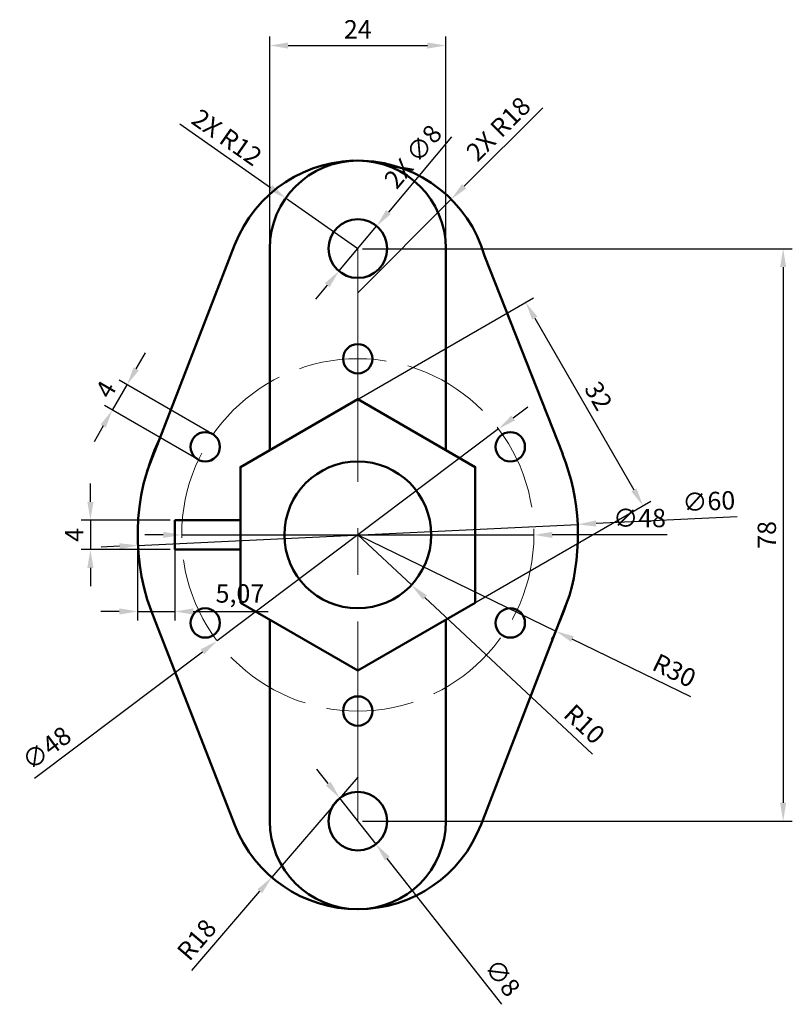
# Model space of a CAD drawing. Units: millimetres. Extents: x 3018 to 3124, y 2213 to 2348.
import ezdxf

# ---------------------------------------------------------------- set-up
doc = ezdxf.new("R2010")
doc.units = ezdxf.units.MM
doc.linetypes.add('ACAD_ISO02W100', pattern=[15, 12, -3])
doc.linetypes.add('CENTER', pattern=[50.8, 31.75, -6.35, 6.35, -6.35])
for name, color, linetype, lineweight in [('M-CNTR', 4, 'CENTER', 18), ('M-CNTR-PCD', 4, 'ACAD_ISO02W100', 18), ('M-DIMS', 2, 'Continuous', 25), ('M-OUTL', 7, 'Continuous', 50)]:
    doc.layers.add(name, color=color, linetype=linetype, lineweight=lineweight)
doc.styles.get("Standard").update_dxf_attribs({"font": 'arial.ttf'})
doc.dimstyles.new('ISO-25', dxfattribs={"dimtxt": 2.5, "dimasz": 2.5, "dimexe": 1.25, "dimexo": 0.625, "dimtad": 1, "dimtxsty": 'Standard', "dimcen": 2.5, "dimadec": 0, "dimazin": 0, "dimtfac": 1, "dimtmove": 0, "dimatfit": 3, "dimfxl": 1, "dimarcsym": 0})

# ---------------------------------------------------------------- blocks, each defined once
blk = doc.blocks.new('*D1')
at = {"layer": 'Defpoints', "color": 0, "transparency": 16777216}
for p in [(3056.3, 2291.27), (3103.18, 2281.39), (3072.3, 2263.56)]:
    blk.add_point(p, dxfattribs=at)
at = {"layer": 'M-DIMS', "color": 0, "lineweight": -2, "transparency": 16777216}
for p, q in [((3056.84, 2291.58), (3088.26, 2309.72)), ((3088.43, 2306.93), (3101.93, 2283.55)), ((3072.84, 2263.87), (3104.26, 2282.01))]:
    blk.add_line(p, q, dxfattribs=at)
at = {"layer": 'M-DIMS', "color": 0, "transparency": 16777216}
for points in [[(3088.79, 2307.14), (3088.07, 2306.73), (3087.18, 2309.1)], [(3102.29, 2283.76), (3101.57, 2283.34), (3103.18, 2281.39)]]:
    blk.add_solid(points, dxfattribs=at)
at = {"layer": 'M-DIMS', "color": 0, "transparency": 16777216, "insert": (3096.83, 2296.19), "char_height": 2.5, "attachment_point": 5, "rotation": 300}
blk.add_mtext('32', dxfattribs=at)
blk = doc.blocks.new('*D2')
at = {"layer": 'Defpoints', "color": 0, "transparency": 16777216}
for p in [(3064.3, 2316.41), (3064.3, 2238.41), (3122.27, 2238.41)]:
    blk.add_point(p, dxfattribs=at)
at = {"layer": 'M-DIMS', "color": 0, "lineweight": -2, "transparency": 16777216}
for p, q in [((3064.93, 2316.41), (3123.52, 2316.41)), ((3122.27, 2313.91), (3122.27, 2240.91)), ((3064.93, 2238.41), (3123.52, 2238.41))]:
    blk.add_line(p, q, dxfattribs=at)
at = {"layer": 'M-DIMS', "color": 0, "transparency": 16777216}
for points in [[(3121.85, 2313.91), (3122.68, 2313.91), (3122.27, 2316.41)], [(3121.85, 2240.91), (3122.68, 2240.91), (3122.27, 2238.41)]]:
    blk.add_solid(points, dxfattribs=at)
at = {"layer": 'M-DIMS', "color": 0, "transparency": 16777216, "insert": (3120.37, 2277.41), "char_height": 2.5, "attachment_point": 5, "rotation": 90}
blk.add_mtext('78', dxfattribs=at)
blk = doc.blocks.new('*D3')
at = {"layer": 'Defpoints', "color": 0, "transparency": 16777216}
for p in [(3076.3, 2344.09), (3052.3, 2316.41), (3076.3, 2316.41)]:
    blk.add_point(p, dxfattribs=at)
at = {"layer": 'M-DIMS', "color": 0, "lineweight": -2, "transparency": 16777216}
for p, q in [((3052.3, 2317.04), (3052.3, 2345.34)), ((3076.3, 2317.04), (3076.3, 2345.34)), ((3054.8, 2344.09), (3073.8, 2344.09))]:
    blk.add_line(p, q, dxfattribs=at)
at = {"layer": 'M-DIMS', "color": 0, "transparency": 16777216}
for points in [[(3054.8, 2344.5), (3054.8, 2343.67), (3052.3, 2344.09)], [(3073.8, 2344.5), (3073.8, 2343.67), (3076.3, 2344.09)]]:
    blk.add_solid(points, dxfattribs=at)
at = {"layer": 'M-DIMS', "color": 0, "transparency": 16777216, "insert": (3064.3, 2345.97), "char_height": 2.5, "attachment_point": 5}
blk.add_mtext('24', dxfattribs=at)
blk = doc.blocks.new('*D4')
at = {"layer": 'Defpoints', "color": 0, "transparency": 16777216}
for p in [(3064.3, 2277.41), (3091.29, 2264.31)]:
    blk.add_point(p, dxfattribs=at)
at = {"layer": 'M-DIMS', "color": 0, "lineweight": -2, "transparency": 16777216}
for p, q in [((3064.3, 2277.41), (3091.29, 2264.31)), ((3109.71, 2255.36), (3093.54, 2263.22))]:
    blk.add_line(p, q, dxfattribs=at)
blk.add_arc((3064.3, 2277.41), 30, 331.7073, 342.802, dxfattribs=at)
at = {"layer": 'M-DIMS', "color": 0, "transparency": 16777216}
blk.add_solid([(3093.72, 2263.59), (3093.36, 2262.84), (3091.29, 2264.31)], dxfattribs=at)
at = {"layer": 'M-DIMS', "color": 0, "transparency": 16777216, "insert": (3107.3, 2258.65), "char_height": 2.5, "attachment_point": 5, "rotation": 334.0946}
blk.add_mtext('R30', dxfattribs=at)
blk = doc.blocks.new('*D5')
at = {"layer": 'Defpoints', "color": 0, "transparency": 16777216}
for p in [(3064.3, 2277.41), (3071.62, 2270.59)]:
    blk.add_point(p, dxfattribs=at)
at = {"layer": 'M-DIMS', "color": 0, "lineweight": -2, "transparency": 16777216}
for p, q in [((3064.3, 2277.41), (3071.62, 2270.59)), ((3096.31, 2247.55), (3073.44, 2268.89))]:
    blk.add_line(p, q, dxfattribs=at)
at = {"layer": 'M-DIMS', "color": 0, "transparency": 16777216}
blk.add_solid([(3073.73, 2269.19), (3073.16, 2268.58), (3071.62, 2270.59)], dxfattribs=at)
at = {"layer": 'M-DIMS', "color": 0, "transparency": 16777216, "insert": (3094.97, 2251.4), "char_height": 2.5, "attachment_point": 5, "rotation": 316.988}
blk.add_mtext('R10', dxfattribs=at)
blk = doc.blocks.new('*D6')
at = {"layer": 'Defpoints', "color": 0, "transparency": 16777216}
for p in [(3061.83, 2241.56), (3066.78, 2235.27)]:
    blk.add_point(p, dxfattribs=at)
at = {"layer": 'M-DIMS', "color": 0, "lineweight": -2, "transparency": 16777216}
for p, q in [((3060.28, 2243.52), (3058.74, 2245.49)), ((3061.83, 2241.56), (3066.78, 2235.27)), ((3083.95, 2213.46), (3068.32, 2233.31))]:
    blk.add_line(p, q, dxfattribs=at)
at = {"layer": 'M-DIMS', "color": 0, "transparency": 16777216}
for points in [[(3060.61, 2243.78), (3059.95, 2243.26), (3061.83, 2241.56)], [(3068.65, 2233.57), (3068, 2233.05), (3066.78, 2235.27)]]:
    blk.add_solid(points, dxfattribs=at)
at = {"layer": 'M-DIMS', "color": 0, "transparency": 16777216, "insert": (3083.77, 2216.88), "char_height": 2.5, "attachment_point": 5, "rotation": 308.2152}
blk.add_mtext('∅8', dxfattribs=at)
blk = doc.blocks.new('*D7')
at = {"layer": 'Defpoints', "color": 0, "transparency": 16777216}
for p in [(3064.3, 2244.41), (3052.58, 2230.76)]:
    blk.add_point(p, dxfattribs=at)
at = {"layer": 'M-DIMS', "color": 0, "lineweight": -2, "transparency": 16777216}
for p, q in [((3064.3, 2244.41), (3052.58, 2230.76)), ((3041.68, 2218.07), (3050.95, 2228.86))]:
    blk.add_line(p, q, dxfattribs=at)
at = {"layer": 'M-DIMS', "color": 0, "transparency": 16777216}
blk.add_solid([(3050.63, 2229.13), (3051.26, 2228.59), (3052.58, 2230.76)], dxfattribs=at)
at = {"layer": 'M-DIMS', "color": 0, "transparency": 16777216, "insert": (3042.59, 2222.05), "char_height": 2.5, "attachment_point": 5, "rotation": 49.3469}
blk.add_mtext('R18', dxfattribs=at)
blk = doc.blocks.new('*D8')
at = {"layer": 'Defpoints', "color": 0, "transparency": 16777216}
for p in [(3039.37, 2279.41), (3027.87, 2275.41), (3039.37, 2275.41)]:
    blk.add_point(p, dxfattribs=at)
at = {"layer": 'M-DIMS', "color": 0, "lineweight": -2, "transparency": 16777216}
for p, q in [((3027.87, 2281.91), (3027.87, 2284.41)), ((3038.74, 2279.41), (3026.62, 2279.41)), ((3027.87, 2279.41), (3027.87, 2275.41)), ((3038.74, 2275.41), (3026.62, 2275.41)), ((3027.87, 2272.91), (3027.87, 2270.41))]:
    blk.add_line(p, q, dxfattribs=at)
at = {"layer": 'M-DIMS', "color": 0, "transparency": 16777216}
for points in [[(3027.45, 2281.91), (3028.28, 2281.91), (3027.87, 2279.41)], [(3027.45, 2272.91), (3028.28, 2272.91), (3027.87, 2275.41)]]:
    blk.add_solid(points, dxfattribs=at)
at = {"layer": 'M-DIMS', "color": 0, "transparency": 16777216, "insert": (3025.99, 2277.41), "char_height": 2.5, "attachment_point": 5, "rotation": 90}
blk.add_mtext('4', dxfattribs=at)
blk = doc.blocks.new('*D9')
at = {"layer": 'Defpoints', "color": 0, "transparency": 16777216}
for p in [(3034.3, 2277.41), (3039.37, 2277.41), (3039.37, 2266.98)]:
    blk.add_point(p, dxfattribs=at)
at = {"layer": 'M-DIMS', "color": 0, "lineweight": -2, "transparency": 16777216}
for p, q in [((3034.3, 2276.79), (3034.3, 2265.73)), ((3039.37, 2276.79), (3039.37, 2265.73)), ((3031.8, 2266.98), (3029.3, 2266.98)), ((3034.3, 2266.98), (3039.37, 2266.98)), ((3041.87, 2266.98), (3052.11, 2266.98))]:
    blk.add_line(p, q, dxfattribs=at)
at = {"layer": 'M-DIMS', "color": 0, "transparency": 16777216}
for points in [[(3031.8, 2267.4), (3031.8, 2266.57), (3034.3, 2266.98)], [(3041.87, 2267.4), (3041.87, 2266.57), (3039.37, 2266.98)]]:
    blk.add_solid(points, dxfattribs=at)
at = {"layer": 'M-DIMS', "color": 0, "transparency": 16777216, "insert": (3048.24, 2269.11), "char_height": 2.5, "attachment_point": 5}
blk.add_mtext('5,07', dxfattribs=at)
blk = doc.blocks.new('*D10')
at = {"layer": 'Defpoints', "color": 0, "transparency": 16777216}
for p in [(3032.86, 2297.88), (3044.59, 2291.1), (3042.59, 2287.64)]:
    blk.add_point(p, dxfattribs=at)
at = {"layer": 'M-DIMS', "color": 0, "lineweight": -2, "transparency": 16777216}
for p, q in [((3034.11, 2300.04), (3035.36, 2302.21)), ((3044.05, 2291.42), (3031.78, 2298.5)), ((3030.86, 2294.42), (3032.86, 2297.88)), ((3042.05, 2287.96), (3029.78, 2295.04)), ((3029.61, 2292.25), (3028.36, 2290.09))]:
    blk.add_line(p, q, dxfattribs=at)
at = {"layer": 'M-DIMS', "color": 0, "transparency": 16777216}
for points in [[(3033.75, 2300.25), (3034.47, 2299.83), (3032.86, 2297.88)], [(3029.25, 2292.46), (3029.97, 2292.04), (3030.86, 2294.42)]]:
    blk.add_solid(points, dxfattribs=at)
at = {"layer": 'M-DIMS', "color": 0, "transparency": 16777216, "insert": (3030.24, 2297.08), "char_height": 2.5, "attachment_point": 5, "rotation": 60}
blk.add_mtext('4', dxfattribs=at)
blk = doc.blocks.new('*D11')
at = {"layer": 'Defpoints', "color": 0, "transparency": 16777216}
for p in [(3083.48, 2291.85), (3045.13, 2262.98)]:
    blk.add_point(p, dxfattribs=at)
at = {"layer": 'M-DIMS', "color": 0, "lineweight": -2, "transparency": 16777216}
for p, q in [((3085.48, 2293.35), (3087.47, 2294.85)), ((3083.48, 2291.85), (3045.13, 2262.98)), ((3020.26, 2244.26), (3043.13, 2261.48))]:
    blk.add_line(p, q, dxfattribs=at)
at = {"layer": 'M-DIMS', "color": 0, "transparency": 16777216}
for points in [[(3085.23, 2293.68), (3085.73, 2293.02), (3083.48, 2291.85)], [(3042.88, 2261.81), (3043.38, 2261.15), (3045.13, 2262.98)]]:
    blk.add_solid(points, dxfattribs=at)
at = {"layer": 'M-DIMS', "color": 0, "transparency": 16777216, "insert": (3022.09, 2248.11), "char_height": 2.5, "attachment_point": 5, "rotation": 36.966}
blk.add_mtext('∅48', dxfattribs=at)
blk = doc.blocks.new('BOLT-HOLE-D4')
blk.add_circle((2, 2), 2)
blk = doc.blocks.new('MOUNT-HOLE-D8')
blk.add_circle((4, 4), 4)
blk = doc.blocks.new('*D14')
at = {"layer": 'Defpoints', "color": 0, "transparency": 16777216}
for p in [(3054.47, 2323.3), (3064.3, 2316.41)]:
    blk.add_point(p, dxfattribs=at)
at = {"layer": 'M-DIMS', "color": 0, "lineweight": -2, "transparency": 16777216}
for p, q in [((3040.05, 2333.4), (3052.43, 2324.73)), ((3064.3, 2316.41), (3054.47, 2323.3))]:
    blk.add_line(p, q, dxfattribs=at)
at = {"layer": 'M-DIMS', "color": 0, "transparency": 16777216}
blk.add_solid([(3052.66, 2325.07), (3052.19, 2324.39), (3054.47, 2323.3)], dxfattribs=at)
at = {"layer": 'M-DIMS', "color": 0, "transparency": 16777216, "insert": (3046.29, 2331.32), "char_height": 2.5, "attachment_point": 5, "rotation": 325.0004}
blk.add_mtext('2X R12', dxfattribs=at)
blk = doc.blocks.new('*D15')
at = {"layer": 'Defpoints', "color": 0, "transparency": 16777216}
for p in [(3094.27, 2278.84), (3034.34, 2275.99)]:
    blk.add_point(p, dxfattribs=at)
at = {"layer": 'M-DIMS', "color": 0, "lineweight": -2, "transparency": 16777216}
for p, q in [((3116.02, 2279.88), (3096.77, 2278.96)), ((3034.34, 2275.99), (3094.27, 2278.84)), ((3031.84, 2275.87), (3029.34, 2275.75))]:
    blk.add_line(p, q, dxfattribs=at)
at = {"layer": 'M-DIMS', "color": 0, "transparency": 16777216}
for points in [[(3096.75, 2279.38), (3096.79, 2278.55), (3094.27, 2278.84)], [(3031.82, 2276.28), (3031.86, 2275.45), (3034.34, 2275.99)]]:
    blk.add_solid(points, dxfattribs=at)
at = {"layer": 'M-DIMS', "color": 0, "transparency": 16777216, "insert": (3112.15, 2281.67), "char_height": 2.5, "attachment_point": 5, "rotation": 2.7282}
blk.add_mtext('∅60', dxfattribs=at)
blk = doc.blocks.new('*D16')
at = {"layer": 'Defpoints', "color": 0, "transparency": 16777216}
for p in [(3040.3, 2277.41), (3088.3, 2277.41)]:
    blk.add_point(p, dxfattribs=at)
at = {"layer": 'M-DIMS', "color": 0, "lineweight": -2, "transparency": 16777216}
for p, q in [((3037.8, 2277.41), (3035.3, 2277.41)), ((3040.3, 2277.41), (3088.3, 2277.41)), ((3106.48, 2277.41), (3090.8, 2277.41))]:
    blk.add_line(p, q, dxfattribs=at)
at = {"layer": 'M-DIMS', "color": 0, "transparency": 16777216}
for points in [[(3037.8, 2277.83), (3037.8, 2277), (3040.3, 2277.41)], [(3090.8, 2277.83), (3090.8, 2277), (3088.3, 2277.41)]]:
    blk.add_solid(points, dxfattribs=at)
at = {"layer": 'M-DIMS', "color": 0, "transparency": 16777216, "insert": (3102.7, 2279.39), "char_height": 2.5, "attachment_point": 5, "rotation": 0}
blk.add_mtext('∅48', dxfattribs=at)
blk = doc.blocks.new('*D17')
at = {"layer": 'Defpoints', "color": 0, "transparency": 16777216}
for p in [(3077.03, 2323.14), (3064.3, 2310.41)]:
    blk.add_point(p, dxfattribs=at)
at = {"layer": 'M-DIMS', "color": 0, "lineweight": -2, "transparency": 16777216}
for p, q in [((3089.51, 2335.62), (3078.8, 2324.91)), ((3064.3, 2310.41), (3077.03, 2323.14))]:
    blk.add_line(p, q, dxfattribs=at)
at = {"layer": 'M-DIMS', "color": 0, "transparency": 16777216}
blk.add_solid([(3078.51, 2325.2), (3079.09, 2324.61), (3077.03, 2323.14)], dxfattribs=at)
at = {"layer": 'M-DIMS', "color": 0, "transparency": 16777216, "insert": (3083.69, 2332.49), "char_height": 2.5, "attachment_point": 5, "rotation": 44.9957}
blk.add_mtext('2X R18', dxfattribs=at)
blk = doc.blocks.new('*D18')
at = {"layer": 'Defpoints', "color": 0, "transparency": 16777216}
for p in [(3066.87, 2319.48), (3061.73, 2313.35)]:
    blk.add_point(p, dxfattribs=at)
at = {"layer": 'M-DIMS', "color": 0, "lineweight": -2, "transparency": 16777216}
for p, q in [((3077.08, 2331.67), (3068.48, 2321.4)), ((3061.73, 2313.35), (3066.87, 2319.48)), ((3060.13, 2311.43), (3058.52, 2309.52))]:
    blk.add_line(p, q, dxfattribs=at)
at = {"layer": 'M-DIMS', "color": 0, "transparency": 16777216}
for points in [[(3068.16, 2321.67), (3068.8, 2321.13), (3066.87, 2319.48)], [(3059.81, 2311.7), (3060.45, 2311.16), (3061.73, 2313.35)]]:
    blk.add_solid(points, dxfattribs=at)
at = {"layer": 'M-DIMS', "color": 0, "transparency": 16777216, "insert": (3072.07, 2328.76), "char_height": 2.5, "attachment_point": 5, "rotation": 50.0542}
blk.add_mtext('2X ∅8', dxfattribs=at)

msp = doc.modelspace()

# ---------------------------------------------------------------- linework, layer by layer
at = {"layer": 'M-CNTR'}
for p, q in [((3064.303, 2316.415), (3064.303, 2238.415)), ((3064.303, 2301.415), (3064.303, 2310.415)), ((3064.303, 2253.415), (3064.303, 2244.415))]:
    msp.add_line(p, q, dxfattribs=at)
at = {"layer": 'M-CNTR-PCD'}
msp.add_circle((3064.303, 2277.415), 24, dxfattribs=at)
at = {"layer": 'M-OUTL'}
for p, q in [((3037.278, 2290.439), (3047.515, 2316.908)), ((3052.303, 2316.415), (3052.303, 2288.962)), ((3076.303, 2316.415), (3076.303, 2288.962)), ((3081.584, 2315.453), (3092.223, 2288.392)), ((3037.278, 2290.439), (3035.601, 2286.145)), ((3048.303, 2279.415), (3039.37, 2279.415)), ((3039.37, 2275.415), (3039.37, 2279.415)), ((3048.303, 2277.415), (3048.303, 2279.415)), ((3048.303, 2277.415), (3048.303, 2275.415)), ((3048.303, 2275.415), (3039.37, 2275.415)), ((3093.14, 2269.144), (3081.096, 2237.934)), ((3052.303, 2265.868), (3052.303, 2238.415)), ((3076.303, 2265.868), (3076.303, 2238.415)), ((3036.733, 2265.588), (3047.532, 2237.879))]:
    msp.add_line(p, q, dxfattribs=at)
msp.add_lwpolyline([(3048.303, 2268.177), (3064.303, 2258.94), (3080.303, 2268.177), (3080.303, 2286.653), (3064.303, 2295.89), (3048.303, 2286.653)], close=True, dxfattribs=at)
msp.add_circle((3064.303, 2277.415), 10, dxfattribs=at)
for centre, radius, start, end in [((3064.303, 2310.415), 18, 16.25207, 158.85521), ((3064.303, 2316.415), 12, 0, 180), ((3064.303, 2277.415), 30, 154.26929, 203.21718), ((3064.303, 2277.415), 30, 343.99565, 21.46237), ((3064.303, 2244.415), 18, 201.29213, 338.89736), ((3064.303, 2238.415), 12, 180, 0)]:
    msp.add_arc(centre, radius, start, end, dxfattribs=at)

# ---------------------------------------------------------------- block references
for name, p in [('MOUNT-HOLE-D8', (3060.303, 2312.415)), ('BOLT-HOLE-D4', (3062.303, 2299.415)), ('BOLT-HOLE-D4', (3041.518, 2287.415)), ('BOLT-HOLE-D4', (3083.088, 2287.415)), ('BOLT-HOLE-D4', (3041.518, 2263.415)), ('BOLT-HOLE-D4', (3083.088, 2263.415)), ('BOLT-HOLE-D4', (3062.303, 2251.415)), ('MOUNT-HOLE-D8', (3060.303, 2234.415))]:
    msp.add_blockref(name, p, dxfattribs=at)

# ---------------------------------------------------------------- dimensions: what is measured, and where the dimension line sits
at = {"layer": 'M-DIMS'}
for base, p1, p2, picture, middle in [((3076.303, 2344.087), (3052.303, 2316.415), (3076.303, 2316.415), '*D3', (3064.303, 2345.967)), ((3039.37, 2266.985), (3034.303, 2277.415), (3039.37, 2277.415), '*D9', (3048.242, 2269.112))]:
    dim = msp.add_linear_dim(base=base, p1=p1, p2=p2, dimstyle='ISO-25', override={"dimclrd": 0, "dimclre": 0, "dimclrt": 0}, dxfattribs=at)
    dim.commit()
    dim.dimension.update_dxf_attribs({"geometry": picture, "text_midpoint": middle})
for center, mpoint, picture, middle in [((3064.303, 2310.415), (3077.032, 2323.142), '*D17', (3083.694, 2332.492)), ((3064.303, 2316.415), (3054.473, 2323.298), '*D14', (3046.29, 2331.324))]:
    dim = msp.add_radius_dim(center=center, mpoint=mpoint, text='2X <>', dimstyle='ISO-25', override={"dimdec": 0, "dimlfac": 1, "dimrnd": 0, "dimzin": 0, "dimdsep": 46, "dimlunit": 2}, dxfattribs=at)
    dim.commit()
    dim.dimension.update_dxf_attribs({"geometry": picture, "text_midpoint": middle})
dim = msp.add_diameter_dim_2p(p1=(3061.735, 2313.348), p2=(3066.871, 2319.482), text='2X <>', dimstyle='ISO-25', override={"dimdec": 0, "dimlfac": 1, "dimrnd": 0, "dimzin": 0, "dimdsep": 46, "dimlunit": 2}, dxfattribs=at)
dim.commit()
dim.dimension.update_dxf_attribs({"geometry": '*D18', "text_midpoint": (3073.579, 2327.491)})
for base, p1, p2, picture, middle in [((3122.268, 2238.415), (3064.303, 2316.415), (3064.303, 2238.415), '*D2', (3120.366, 2277.415)), ((3027.867, 2275.415), (3039.37, 2279.415), (3039.37, 2275.415), '*D8', (3025.992, 2277.415))]:
    dim = msp.add_linear_dim(base=base, p1=p1, p2=p2, angle=90, dimstyle='ISO-25', override={"dimclrd": 0, "dimclre": 0, "dimclrt": 0}, dxfattribs=at)
    dim.commit()
    dim.dimension.update_dxf_attribs({"geometry": picture, "text_midpoint": middle})
for p1, p2, distance, picture, middle in [((3056.303, 2291.271), (3072.303, 2263.559), 35.655, '*D1', (3096.829, 2296.194)), ((3042.592, 2287.643), (3044.59, 2291.104), 13.545, '*D10', (3030.236, 2297.083))]:
    dim = msp.add_aligned_dim(p1=p1, p2=p2, distance=distance, dimstyle='ISO-25', override={"dimclrd": 0, "dimclre": 0, "dimclrt": 0}, dxfattribs=at)
    dim.commit()
    dim.dimension.update_dxf_attribs({"geometry": picture, "text_midpoint": middle})
for p1, p2, override, picture, middle in [((3083.479, 2291.847), (3045.127, 2262.983), {"dimclrd": 0, "dimclre": 0, "dimclrt": 0}, '*D11', (3023.276, 2246.537)), ((3034.337, 2275.987), (3094.269, 2278.843), {"dimdec": 0, "dimlfac": 1, "dimrnd": 0, "dimzin": 0, "dimdsep": 46, "dimlunit": 2}, '*D15', (3112.249, 2279.7)), ((3040.303, 2277.415), (3088.303, 2277.415), {"dimdec": 0, "dimlfac": 1, "dimrnd": 0, "dimzin": 0, "dimdsep": 46, "dimlunit": 2}, '*D16', (3102.703, 2277.415)), ((3061.829, 2241.558), (3066.778, 2235.272), {"dimclrd": 0, "dimclre": 0, "dimclrt": 0}, '*D6', (3082.217, 2215.663))]:
    dim = msp.add_diameter_dim_2p(p1=p1, p2=p2, dimstyle='ISO-25', override=override, dxfattribs=at)
    dim.commit()
    dim.dimension.update_dxf_attribs({"geometry": picture, "text_midpoint": middle, "dimtype": 163})
for center, mpoint, picture, middle in [((3064.303, 2277.415), (3091.289, 2264.308), '*D4', (3106.468, 2256.936)), ((3064.303, 2277.415), (3071.615, 2270.593), '*D5', (3093.676, 2250.013)), ((3064.303, 2244.415), (3052.576, 2230.759), '*D7', (3044.036, 2220.813))]:
    dim = msp.add_radius_dim(center=center, mpoint=mpoint, dimstyle='ISO-25', override={"dimclrd": 0, "dimclre": 0, "dimclrt": 0}, dxfattribs=at)
    dim.commit()
    dim.dimension.update_dxf_attribs({"geometry": picture, "text_midpoint": middle, "dimtype": 164})

doc.saveas('drawing.dxf')
